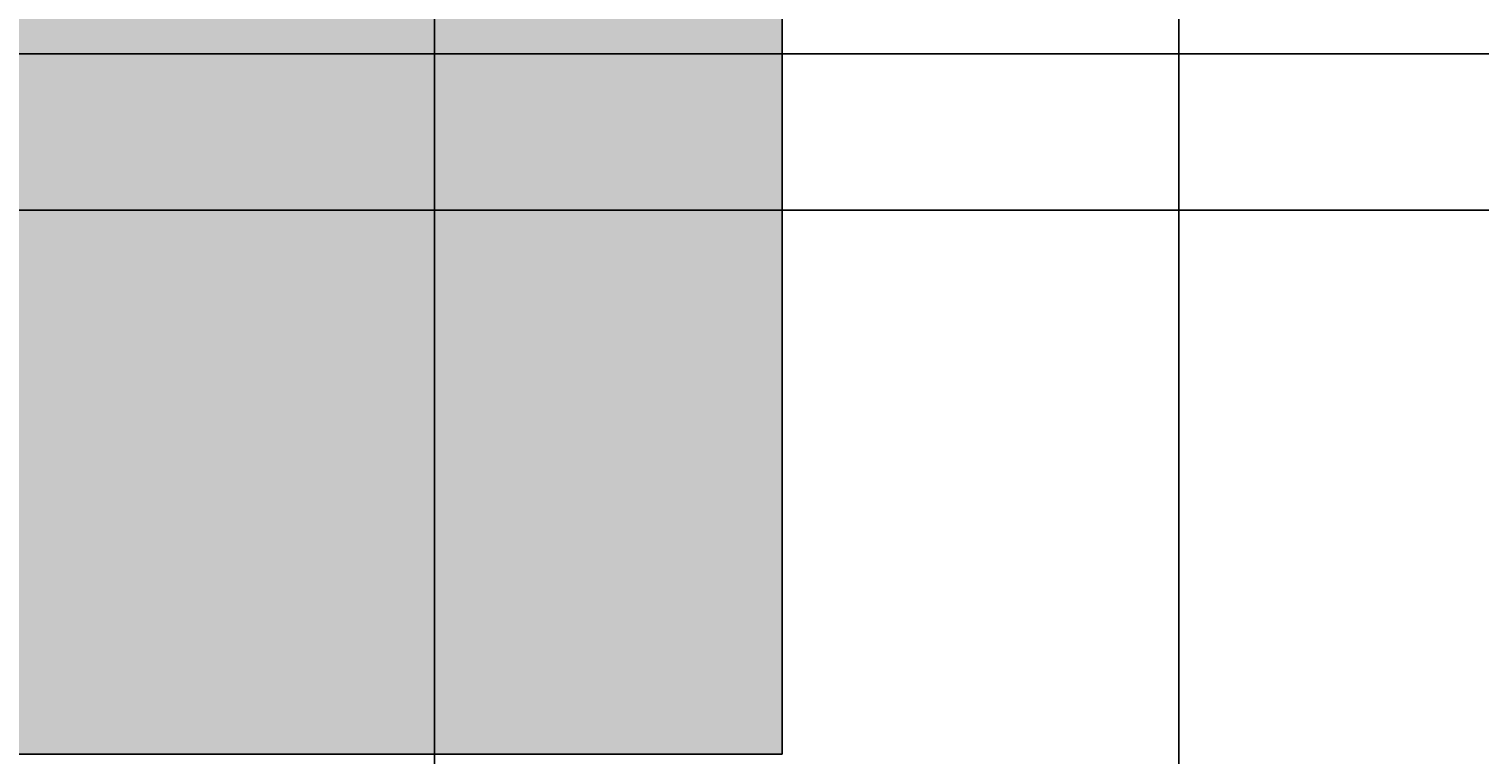
# Model space of a CAD drawing. Units: inches. Extents: x 35362 to 73946, y 43607 to 67532.
# Tile 60 of 134: x 47763 to 48533, y 46919 to 47304. Entities that reach past the tile are written whole.
import ezdxf

# ---------------------------------------------------------------- set-up
doc = ezdxf.new("R2010")
doc.units = ezdxf.units.IN
doc.header["$MEASUREMENT"] = 0
for name, color, linetype, lineweight in [('A-ANNO-DIMS', 2, 'Continuous', 18), ('E-SYMB', 1, 'Continuous', 25), ('E-SYMB-PATT', 1, 'Continuous', 13)]:
    doc.layers.add(name, color=color, linetype=linetype, lineweight=lineweight)
doc.styles.get("Standard").update_dxf_attribs({"font": 'arial.ttf'})
doc.dimstyles.get("Standard").update_dxf_attribs({"dimtxt": 0.18, "dimasz": 0.18, "dimexe": 0.18, "dimexo": 0.0625, "dimgap": 0.09, "dimtad": 0, "dimtih": 1, "dimtoh": 1, "dimdec": 4, "dimzin": 0, "dimdsep": 46, "dimtxsty": 'Standard', "dimcen": 0.09, "dimadec": 0, "dimazin": 0, "dimtfac": 1, "dimtdec": 4, "dimtofl": 0, "dimtmove": 0, "dimatfit": 3, "dimfxl": 1, "dimtolj": 1, "dimtzin": 0, "dimarcsym": 0})

# ---------------------------------------------------------------- blocks, each defined once
blk = doc.blocks.new('*D11')
at = {"layer": 'A-ANNO-DIMS', "color": 0, "lineweight": -2, "transparency": 16777216}
for p, q in [((47978.66, 56028.77), (47978.66, 43606.68)), ((53109.76, 56028.77), (53109.76, 43606.68)), ((47978.84, 43606.86), (50543.87, 43606.86)), ((53109.58, 43606.86), (50544.55, 43606.86))]:
    blk.add_line(p, q, dxfattribs=at)
at = {"layer": 'A-ANNO-DIMS', "color": 0, "transparency": 16777216}
for points in [[(47978.84, 43606.89), (47978.84, 43606.83), (47978.66, 43606.86)], [(53109.58, 43606.89), (53109.58, 43606.83), (53109.76, 43606.86)]]:
    blk.add_solid(points, dxfattribs=at)
at = {"layer": 'Defpoints', "color": 0, "transparency": 16777216}
for p in [(47978.66, 56028.84), (53109.76, 56028.84), (53109.76, 43606.86)]:
    blk.add_point(p, dxfattribs=at)
at = {"layer": 'A-ANNO-DIMS', "color": 0, "transparency": 16777216, "insert": (50544.21, 43606.86), "char_height": 0.18, "attachment_point": 5}
blk.add_mtext('\\A1;5131', dxfattribs=at)
blk = doc.blocks.new('*D13')
at = {"layer": 'A-ANNO-DIMS', "color": 0, "lineweight": -2, "transparency": 16777216}
for p, q in [((48373.49, 51694.02), (48373.49, 43606.68)), ((51029.04, 51694.02), (51029.04, 43606.68)), ((48373.67, 43606.86), (49700.8, 43606.86)), ((51028.86, 43606.86), (49701.73, 43606.86))]:
    blk.add_line(p, q, dxfattribs=at)
at = {"layer": 'A-ANNO-DIMS', "color": 0, "transparency": 16777216}
for points in [[(48373.67, 43606.89), (48373.67, 43606.83), (48373.49, 43606.86)], [(51028.86, 43606.89), (51028.86, 43606.83), (51029.04, 43606.86)]]:
    blk.add_solid(points, dxfattribs=at)
at = {"layer": 'Defpoints', "color": 0, "transparency": 16777216}
for p in [(48373.49, 51694.09), (51029.04, 51694.09), (51029.04, 43606.86)]:
    blk.add_point(p, dxfattribs=at)
at = {"layer": 'A-ANNO-DIMS', "color": 0, "transparency": 16777216, "insert": (49701.27, 43606.86), "char_height": 0.18, "attachment_point": 5}
blk.add_mtext('\\A1;2655.6', dxfattribs=at)
blk = doc.blocks.new('*D27')
at = {"layer": 'A-ANNO-DIMS', "color": 0, "lineweight": -2, "transparency": 16777216}
for p, q in [((47978.66, 56028.77), (47978.66, 43606.68)), ((48373.49, 53428.96), (48373.49, 43606.68)), ((47978.84, 43606.86), (48175.68, 43606.86)), ((48373.31, 43606.86), (48176.47, 43606.86))]:
    blk.add_line(p, q, dxfattribs=at)
at = {"layer": 'A-ANNO-DIMS', "color": 0, "transparency": 16777216}
for points in [[(47978.84, 43606.89), (47978.84, 43606.83), (47978.66, 43606.86)], [(48373.31, 43606.89), (48373.31, 43606.83), (48373.49, 43606.86)]]:
    blk.add_solid(points, dxfattribs=at)
at = {"layer": 'Defpoints', "color": 0, "transparency": 16777216}
for p in [(47978.66, 56028.84), (48373.49, 53429.02), (48373.49, 43606.86)]:
    blk.add_point(p, dxfattribs=at)
at = {"layer": 'A-ANNO-DIMS', "color": 0, "transparency": 16777216, "insert": (48176.08, 43606.86), "char_height": 0.18, "attachment_point": 5}
blk.add_mtext('\\A1;394.8', dxfattribs=at)
blk = doc.blocks.new('*D43')
at = {"layer": 'A-ANNO-DIMS', "color": 0, "lineweight": -2, "transparency": 16777216}
for p, q in [((62004.67, 47625.18), (35361.77, 47625.18)), ((35361.95, 47625), (35361.95, 47416.9)), ((35361.95, 47208.43), (35361.95, 47416.53)), ((62004.67, 47208.25), (35361.77, 47208.25))]:
    blk.add_line(p, q, dxfattribs=at)
at = {"layer": 'A-ANNO-DIMS', "color": 0, "transparency": 16777216}
for points in [[(35361.92, 47625), (35361.98, 47625), (35361.95, 47625.18)], [(35361.92, 47208.43), (35361.98, 47208.43), (35361.95, 47208.25)]]:
    blk.add_solid(points, dxfattribs=at)
at = {"layer": 'Defpoints', "color": 0, "transparency": 16777216}
for p in [(62004.73, 47625.18), (35361.95, 47208.25), (62004.73, 47208.25)]:
    blk.add_point(p, dxfattribs=at)
at = {"layer": 'A-ANNO-DIMS', "color": 0, "transparency": 16777216, "insert": (35361.95, 47416.72), "char_height": 0.18, "attachment_point": 5}
blk.add_mtext('\\A1;416.9', dxfattribs=at)
blk = doc.blocks.new('*D67')
at = {"layer": 'A-ANNO-DIMS', "color": 0, "lineweight": -2, "transparency": 16777216}
for p, q in [((56873.54, 53351.53), (35361.77, 53351.53)), ((35361.95, 53351.35), (35361.95, 49400.89)), ((35361.95, 45450.07), (35361.95, 49400.53)), ((53793.58, 45449.89), (35361.77, 45449.89))]:
    blk.add_line(p, q, dxfattribs=at)
at = {"layer": 'A-ANNO-DIMS', "color": 0, "transparency": 16777216}
for points in [[(35361.92, 53351.35), (35361.98, 53351.35), (35361.95, 53351.53)], [(35361.92, 45450.07), (35361.98, 45450.07), (35361.95, 45449.89)]]:
    blk.add_solid(points, dxfattribs=at)
at = {"layer": 'Defpoints', "color": 0, "transparency": 16777216}
for p in [(35361.95, 53351.53), (56873.6, 53351.53), (53793.64, 45449.89)]:
    blk.add_point(p, dxfattribs=at)
at = {"layer": 'A-ANNO-DIMS', "color": 0, "transparency": 16777216, "insert": (35361.95, 49400.71), "char_height": 0.18, "attachment_point": 5}
blk.add_mtext('\\A1;7901.6', dxfattribs=at)
blk = doc.blocks.new('*D90')
at = {"layer": 'A-ANNO-DIMS', "color": 0, "lineweight": -2, "transparency": 16777216}
for p, q in [((53707.72, 47291.29), (35361.77, 47291.29)), ((35361.95, 47291.11), (35361.95, 46710.26)), ((35361.95, 46129.06), (35361.95, 46709.9)), ((53793.58, 46128.88), (35361.77, 46128.88))]:
    blk.add_line(p, q, dxfattribs=at)
at = {"layer": 'A-ANNO-DIMS', "color": 0, "transparency": 16777216}
for points in [[(35361.92, 47291.11), (35361.98, 47291.11), (35361.95, 47291.29)], [(35361.92, 46129.06), (35361.98, 46129.06), (35361.95, 46128.88)]]:
    blk.add_solid(points, dxfattribs=at)
at = {"layer": 'Defpoints', "color": 0, "transparency": 16777216}
for p in [(53707.78, 47291.29), (35361.95, 46128.88), (53793.64, 46128.88)]:
    blk.add_point(p, dxfattribs=at)
at = {"layer": 'A-ANNO-DIMS', "color": 0, "transparency": 16777216, "insert": (35361.95, 46710.08), "char_height": 0.18, "attachment_point": 5}
blk.add_mtext('\\A1;1162.4', dxfattribs=at)

msp = doc.modelspace()

# ---------------------------------------------------------------- hatches: boundary and pattern name
at = {"layer": 'E-SYMB-PATT'}
h = msp.add_hatch(color=256, dxfattribs=at)
h.dxf.hatch_style = 1
h.paths.add_polyline_path([(48163.038, 49689.843), (45390.147, 49689.843), (45390.147, 46919.381), (48163.038, 46919.381)])

# ---------------------------------------------------------------- linework, layer by layer
at = {"layer": 'E-SYMB'}
msp.add_lwpolyline([(45390.147, 49689.843), (48163.038, 49689.843), (48163.038, 46919.381), (45390.147, 46919.381)], close=True, dxfattribs=at)

# ---------------------------------------------------------------- dimensions: what is measured, and where the dimension line sits
at = {"layer": 'A-ANNO-DIMS'}
for base, p1, p2, override, picture, middle in [((53109.76, 43606.859), (47978.665, 56028.836), (53109.76, 56028.836), {"dimdec": 0, "dimlfac": 1, "dimrnd": 0, "dimzin": 0, "dimdsep": 46, "dimlunit": 2}, '*D11', (50544.212, 43606.859)), ((48373.492, 43606.859), (47978.665, 56028.836), (48373.492, 53429.019), {"dimdec": 1, "dimlfac": 1, "dimrnd": 0, "dimzin": 0, "dimdsep": 46, "dimlunit": 2}, '*D27', (48176.078, 43606.859)), ((51029.043, 43606.859), (48373.492, 51694.087), (51029.043, 51694.087), {"dimdec": 1, "dimlfac": 1, "dimrnd": 0, "dimzin": 0, "dimdsep": 46, "dimlunit": 2}, '*D13', (49701.267, 43606.859))]:
    dim = msp.add_linear_dim(base=base, p1=p1, p2=p2, dimstyle='Standard', override=override, dxfattribs=at)
    dim.commit()
    dim.dimension.update_dxf_attribs({"geometry": picture, "text_midpoint": middle})
for base, p1, p2, picture, middle in [((35361.949, 53351.529), (53793.638, 45449.894), (56873.602, 53351.529), '*D67', (35361.949, 49400.712)), ((35361.949, 47208.25), (62004.728, 47625.181), (62004.728, 47208.25), '*D43', (35361.949, 47416.715)), ((35361.949, 46128.878), (53707.781, 47291.285), (53793.638, 46128.878), '*D90', (35361.949, 46710.081))]:
    dim = msp.add_linear_dim(base=base, p1=p1, p2=p2, angle=90, dimstyle='Standard', override={"dimdec": 1, "dimlfac": 1, "dimrnd": 0, "dimzin": 0, "dimdsep": 46, "dimlunit": 2}, dxfattribs=at)
    dim.commit()
    dim.dimension.update_dxf_attribs({"geometry": picture, "text_midpoint": middle})

doc.saveas('drawing.dxf')
